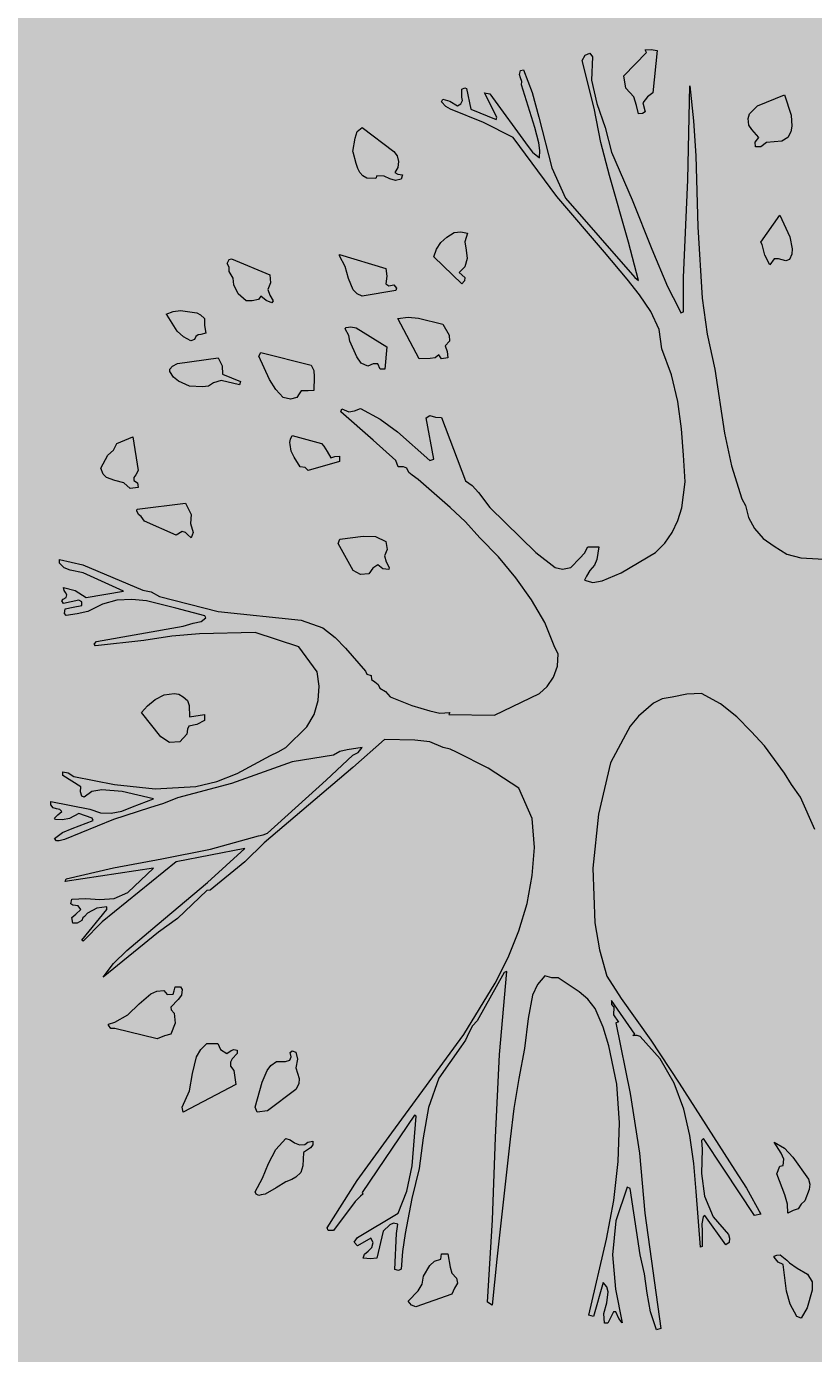
# Model space of a CAD drawing. Units: inches. Extents: x 84 to 1044, y -280 to 906.
# Tile 70 of 105: x 705 to 719, y 408 to 432. Entities that reach past the tile are written whole.
import ezdxf

# ---------------------------------------------------------------- set-up
doc = ezdxf.new("R2010")
doc.units = ezdxf.units.IN
doc.layers.add('A-ANNO-DIMS', color=2, linetype='Continuous', lineweight=18)
doc.layers.add('L-PLNT', color=114, linetype='Continuous', lineweight=15)
doc.layers.add('L-PLNT-PATT', color=9, linetype='Continuous', lineweight=9, true_color=0xafd9aa)
doc.styles.get("Standard").update_dxf_attribs({"font": 'arial.ttf'})
doc.dimstyles.get("Standard").update_dxf_attribs({"dimtxt": 0.18, "dimasz": 0.18, "dimexe": 0.18, "dimexo": 0.0625, "dimgap": 0.09, "dimtad": 0, "dimtih": 1, "dimtoh": 1, "dimdec": 4, "dimzin": 0, "dimdsep": 46, "dimtxsty": 'Standard', "dimcen": 0.09, "dimadec": 0, "dimazin": 0, "dimtfac": 1, "dimtdec": 4, "dimtofl": 0, "dimtmove": 0, "dimatfit": 3, "dimfxl": 1, "dimtolj": 1, "dimtzin": 0, "dimarcsym": 0})

# ---------------------------------------------------------------- blocks, each defined once
blk = doc.blocks.new('A$C37E508DF')
for p, q in [((0.6329, 1.5111), (0.6367, 1.5175)), ((0.6367, 1.5175), (0.6423, 1.5201)), ((0.6423, 1.5201), (0.6453, 1.5158)), ((0.6826, 1.493), (0.7096, 1.5209)), ((0.7083, 1.5239), (0.7152, 1.5244)), ((0.7096, 1.5209), (0.7083, 1.5239)), ((0.7152, 1.5244), (0.7225, 1.5231)), ((0.7225, 1.5231), (0.7174, 1.4729)), ((0.6475, 1.4545), (0.6329, 1.5111)), ((0.6453, 1.5158), (0.644, 1.4879)), ((0.5583, 1.4948), (0.5596, 1.4995)), ((0.5596, 1.4905), (0.5583, 1.4948)), ((0.5596, 1.4995), (0.563, 1.5003)), ((0.5613, 1.4862), (0.5596, 1.4905)), ((0.5608, 1.4823), (0.5613, 1.4862)), ((0.563, 1.5003), (0.5737, 1.4733)), ((0.644, 1.4879), (0.6505, 1.46)), ((0.6852, 1.4785), (0.6826, 1.493)), ((0.4897, 1.4772), (0.4935, 1.4789)), ((0.4897, 1.4678), (0.4897, 1.4772)), ((0.4935, 1.4789), (0.4952, 1.478)), ((0.4952, 1.478), (0.5004, 1.4532)), ((0.5313, 1.4437), (0.5167, 1.4729)), ((0.5167, 1.4729), (0.5231, 1.4716)), ((0.5231, 1.4716), (0.5686, 1.409)), ((0.5767, 1.4317), (0.5608, 1.4823)), ((0.5737, 1.4733), (0.5814, 1.4437)), ((0.6946, 1.4682), (0.6852, 1.4785)), ((0.7174, 1.4729), (0.7109, 1.4682)), ((0.7589, 1.3691), (0.7615, 1.481)), ((0.7615, 1.481), (0.7658, 1.4395)), ((0.8421, 1.4575), (0.8739, 1.4703)), ((0.8739, 1.4703), (0.882, 1.4463)), ((0.4657, 1.4622), (0.4669, 1.4652)), ((0.4708, 1.4566), (0.4657, 1.4622)), ((0.4669, 1.4652), (0.4755, 1.463)), ((0.4764, 1.4532), (0.4708, 1.4566)), ((0.4755, 1.463), (0.4845, 1.4575)), ((0.4845, 1.4575), (0.4884, 1.4596)), ((0.4884, 1.4596), (0.4905, 1.4635)), ((0.4905, 1.4635), (0.4897, 1.4678)), ((0.6552, 1.4137), (0.6475, 1.4545)), ((0.6505, 1.46), (0.6603, 1.4317)), ((0.6976, 1.4579), (0.6946, 1.4682)), ((0.7002, 1.4476), (0.6976, 1.4579)), ((0.7109, 1.4682), (0.7053, 1.4609)), ((0.7053, 1.4609), (0.7083, 1.4502)), ((0.8357, 1.451), (0.8421, 1.4575)), ((0.5154, 1.4373), (0.4764, 1.4532)), ((0.5004, 1.4532), (0.5308, 1.4412)), ((0.5308, 1.4412), (0.5313, 1.4437)), ((0.5814, 1.4437), (0.5969, 1.3833)), ((0.7049, 1.448), (0.7002, 1.4476)), ((0.7083, 1.4502), (0.7049, 1.448)), ((0.7658, 1.4395), (0.7684, 1.3979)), ((0.831, 1.4424), (0.8323, 1.4476)), ((0.8318, 1.4343), (0.831, 1.4424)), ((0.8323, 1.4476), (0.8357, 1.451)), ((0.882, 1.4463), (0.8829, 1.433)), ((0.3628, 1.4189), (0.3649, 1.4266)), ((0.3649, 1.4266), (0.3709, 1.4317)), ((0.3709, 1.4317), (0.4086, 1.403)), ((0.551, 1.4197), (0.5154, 1.4373)), ((0.5814, 1.4133), (0.5767, 1.4317)), ((0.6603, 1.4317), (0.668, 1.4021)), ((0.8353, 1.4292), (0.8318, 1.4343)), ((0.8434, 1.4197), (0.8353, 1.4292)), ((0.8816, 1.4262), (0.8781, 1.4197)), ((0.8829, 1.433), (0.8816, 1.4262)), ((0.3598, 1.403), (0.3628, 1.4189)), ((0.6029, 1.3494), (0.551, 1.4197)), ((0.5686, 1.409), (0.5741, 1.4021)), ((0.5827, 1.4043), (0.5814, 1.4133)), ((0.6655, 1.3743), (0.6552, 1.4137)), ((0.8391, 1.4141), (0.8434, 1.4197)), ((0.8395, 1.4086), (0.8391, 1.4141)), ((0.846, 1.4086), (0.8395, 1.4086)), ((0.8528, 1.4137), (0.846, 1.4086)), ((0.8619, 1.4146), (0.8528, 1.4137)), ((0.8709, 1.4154), (0.8619, 1.4146)), ((0.8781, 1.4197), (0.8709, 1.4154)), ((0.3602, 1.4021), (0.3598, 1.403)), ((0.364, 1.3888), (0.3602, 1.4021)), ((0.4086, 1.403), (0.4125, 1.3979)), ((0.4125, 1.3979), (0.4142, 1.391)), ((0.4142, 1.391), (0.4134, 1.3837)), ((0.5741, 1.4021), (0.5823, 1.3953)), ((0.5823, 1.3953), (0.5827, 1.4043)), ((0.668, 1.4021), (0.6925, 1.3455)), ((0.7684, 1.3979), (0.771, 1.3134)), ((0.3657, 1.3828), (0.364, 1.3888)), ((0.3683, 1.3781), (0.3657, 1.3828)), ((0.3718, 1.3738), (0.3683, 1.3781)), ((0.4134, 1.3837), (0.4099, 1.3781)), ((0.4099, 1.3781), (0.4134, 1.376)), ((0.4134, 1.376), (0.4189, 1.3751)), ((0.4189, 1.3751), (0.4176, 1.37)), ((0.5969, 1.3833), (0.6132, 1.3472)), ((0.3765, 1.3713), (0.3718, 1.3738)), ((0.3872, 1.3708), (0.3765, 1.3713)), ((0.3885, 1.3738), (0.3872, 1.3708)), ((0.3971, 1.3734), (0.3885, 1.3738)), ((0.4039, 1.3704), (0.3971, 1.3734)), ((0.4108, 1.3683), (0.4039, 1.3704)), ((0.4176, 1.37), (0.4108, 1.3683)), ((0.6882, 1.2949), (0.6655, 1.3743)), ((0.7538, 1.2529), (0.7589, 1.3691)), ((0.6595, 1.2829), (0.6029, 1.3494)), ((0.6132, 1.3472), (0.6959, 1.2529)), ((0.6925, 1.3455), (0.7161, 1.2868)), ((0.771, 1.3134), (0.7761, 1.2285)), ((0.846, 1.2949), (0.8687, 1.3271)), ((0.8687, 1.3271), (0.8803, 1.3014)), ((0.4648, 1.2945), (0.4717, 1.3009)), ((0.4717, 1.3009), (0.4807, 1.3065)), ((0.4807, 1.3065), (0.4884, 1.3074)), ((0.4884, 1.3074), (0.4965, 1.3057)), ((0.4965, 1.3057), (0.4935, 1.2954)), ((0.8803, 1.3014), (0.8833, 1.2872)), ((0.3439, 1.2804), (0.3992, 1.2636)), ((0.3439, 1.2787), (0.3439, 1.2804)), ((0.4562, 1.2774), (0.4597, 1.2868)), ((0.4597, 1.2868), (0.4648, 1.2945)), ((0.4935, 1.2954), (0.4948, 1.2855)), ((0.4948, 1.2855), (0.4961, 1.2756)), ((0.6865, 1.2508), (0.6595, 1.2829)), ((0.7002, 1.2495), (0.6882, 1.2949)), ((0.7161, 1.2868), (0.7349, 1.2422)), ((0.8473, 1.2924), (0.846, 1.2949)), ((0.8507, 1.2795), (0.8473, 1.2924)), ((0.8829, 1.2808), (0.8799, 1.2744)), ((0.8833, 1.2872), (0.8829, 1.2808)), ((0.2101, 1.2696), (0.2127, 1.2744)), ((0.2127, 1.2654), (0.2101, 1.2696)), ((0.2127, 1.2744), (0.2152, 1.2752)), ((0.2127, 1.2602), (0.2127, 1.2654)), ((0.2152, 1.2752), (0.2611, 1.2559)), ((0.3507, 1.2662), (0.3439, 1.2787)), ((0.3546, 1.2516), (0.3507, 1.2662)), ((0.4897, 1.2452), (0.4562, 1.2774)), ((0.4935, 1.2658), (0.4867, 1.2589)), ((0.4961, 1.2756), (0.4935, 1.2658)), ((0.8567, 1.2679), (0.8507, 1.2795)), ((0.8619, 1.2752), (0.8567, 1.2679)), ((0.867, 1.2752), (0.8619, 1.2752)), ((0.8713, 1.2739), (0.867, 1.2752)), ((0.8756, 1.2726), (0.8713, 1.2739)), ((0.8799, 1.2744), (0.8756, 1.2726)), ((0.2174, 1.2521), (0.2127, 1.2602)), ((0.2182, 1.2443), (0.2174, 1.2521)), ((0.2611, 1.2559), (0.262, 1.2465)), ((0.3602, 1.2383), (0.3546, 1.2516)), ((0.3992, 1.2636), (0.4005, 1.2546)), ((0.4005, 1.2546), (0.3992, 1.2452)), ((0.4867, 1.2589), (0.4935, 1.2529)), ((0.4931, 1.2491), (0.4897, 1.2452)), ((0.4935, 1.2529), (0.4931, 1.2491)), ((0.7015, 1.2323), (0.6865, 1.2508)), ((0.6959, 1.2529), (0.7002, 1.2495)), ((0.7538, 1.2122), (0.7538, 1.2529)), ((0.2234, 1.2336), (0.2182, 1.2443)), ((0.2328, 1.2251), (0.2234, 1.2336)), ((0.262, 1.2465), (0.2586, 1.2388)), ((0.2586, 1.2388), (0.2611, 1.2319)), ((0.3649, 1.2336), (0.3602, 1.2383)), ((0.3709, 1.2306), (0.3649, 1.2336)), ((0.4112, 1.2375), (0.3709, 1.2306)), ((0.3992, 1.2452), (0.4026, 1.2431)), ((0.4026, 1.2431), (0.4086, 1.2443)), ((0.4086, 1.2443), (0.4121, 1.2401)), ((0.4121, 1.2401), (0.4112, 1.2375)), ((0.7349, 1.2422), (0.7482, 1.216)), ((0.2401, 1.2251), (0.2328, 1.2251)), ((0.2474, 1.2268), (0.2401, 1.2251)), ((0.2504, 1.2306), (0.2474, 1.2268)), ((0.2568, 1.2255), (0.2504, 1.2306)), ((0.2633, 1.2229), (0.2568, 1.2255)), ((0.2611, 1.2319), (0.265, 1.2251)), ((0.265, 1.2251), (0.2633, 1.2229)), ((0.7148, 1.2126), (0.7015, 1.2323)), ((0.7761, 1.2285), (0.7821, 1.1856)), ((0.1376, 1.2092), (0.1458, 1.2126)), ((0.1389, 1.2079), (0.1376, 1.2092)), ((0.1505, 1.189), (0.1389, 1.2079)), ((0.1458, 1.2126), (0.1548, 1.2135)), ((0.1548, 1.2135), (0.1741, 1.2109)), ((0.1741, 1.2109), (0.1784, 1.2083)), ((0.1784, 1.2083), (0.1831, 1.204)), ((0.1831, 1.204), (0.1831, 1.1959)), ((0.4134, 1.204), (0.4258, 1.2058)), ((0.4391, 1.156), (0.4134, 1.204)), ((0.4258, 1.2058), (0.4382, 1.2045)), ((0.4382, 1.2045), (0.4669, 1.1972)), ((0.7246, 1.1908), (0.7148, 1.2126)), ((0.7482, 1.216), (0.7508, 1.2109)), ((0.7508, 1.2109), (0.7538, 1.2122)), ((0.1582, 1.1822), (0.1505, 1.189)), ((0.1788, 1.1852), (0.1758, 1.1847)), ((0.1848, 1.1865), (0.1788, 1.1852)), ((0.1831, 1.1959), (0.1848, 1.1865)), ((0.3507, 1.1916), (0.352, 1.1933)), ((0.355, 1.1839), (0.3507, 1.1916)), ((0.352, 1.1933), (0.3576, 1.1942)), ((0.3576, 1.1942), (0.364, 1.1929)), ((0.364, 1.1929), (0.4005, 1.1702)), ((0.4669, 1.1972), (0.4747, 1.1843)), ((0.7281, 1.168), (0.7246, 1.1908)), ((0.7821, 1.1856), (0.7911, 1.1436)), ((0.1668, 1.1775), (0.1582, 1.1822)), ((0.1711, 1.1792), (0.1668, 1.1775)), ((0.1728, 1.1826), (0.1711, 1.1792)), ((0.1758, 1.1847), (0.1728, 1.1826)), ((0.3563, 1.177), (0.355, 1.1839)), ((0.3645, 1.1586), (0.3563, 1.177)), ((0.4005, 1.1702), (0.3979, 1.1436)), ((0.4751, 1.177), (0.47, 1.1714)), ((0.47, 1.1714), (0.4721, 1.1646)), ((0.4747, 1.1843), (0.4751, 1.177)), ((0.1509, 1.1504), (0.1994, 1.1573)), ((0.1994, 1.1573), (0.2041, 1.1479)), ((0.2478, 1.1594), (0.2504, 1.1637)), ((0.2607, 1.1316), (0.2478, 1.1594)), ((0.2504, 1.1637), (0.3104, 1.1487)), ((0.37, 1.1509), (0.3645, 1.1586)), ((0.4519, 1.1564), (0.4391, 1.156)), ((0.458, 1.1573), (0.4519, 1.1564)), ((0.4622, 1.1607), (0.458, 1.1573)), ((0.4657, 1.156), (0.4622, 1.1607)), ((0.473, 1.1573), (0.4657, 1.156)), ((0.4721, 1.1646), (0.473, 1.1573)), ((0.7396, 1.1371), (0.7281, 1.168)), ((0.1419, 1.1436), (0.1449, 1.1474)), ((0.1419, 1.141), (0.1419, 1.1436)), ((0.1462, 1.1342), (0.1419, 1.141)), ((0.1449, 1.1474), (0.1509, 1.1504)), ((0.2041, 1.1479), (0.2045, 1.138)), ((0.2045, 1.138), (0.226, 1.129)), ((0.3104, 1.1487), (0.3134, 1.1423)), ((0.3134, 1.1423), (0.3139, 1.1346)), ((0.3778, 1.1474), (0.37, 1.1509)), ((0.3842, 1.15), (0.3778, 1.1474)), ((0.3898, 1.15), (0.3842, 1.15)), ((0.3923, 1.1436), (0.3898, 1.15)), ((0.3979, 1.1436), (0.3923, 1.1436)), ((0.7911, 1.1436), (0.8027, 1.0677)), ((0.1522, 1.1294), (0.1462, 1.1342)), ((0.1655, 1.1234), (0.1522, 1.1294)), ((0.181, 1.1226), (0.1655, 1.1234)), ((0.1878, 1.1234), (0.181, 1.1226)), ((0.1938, 1.1273), (0.1878, 1.1234)), ((0.2032, 1.1303), (0.1938, 1.1273)), ((0.2247, 1.1251), (0.2032, 1.1303)), ((0.226, 1.129), (0.2247, 1.1251)), ((0.268, 1.1196), (0.2607, 1.1316)), ((0.3139, 1.1346), (0.3134, 1.1183)), ((0.7469, 1.1054), (0.7396, 1.1371)), ((0.277, 1.1101), (0.268, 1.1196)), ((0.2856, 1.108), (0.277, 1.1101)), ((0.2933, 1.1101), (0.2856, 1.108)), ((0.2959, 1.1144), (0.2933, 1.1101)), ((0.2984, 1.1179), (0.2959, 1.1144)), ((0.3066, 1.1179), (0.2984, 1.1179)), ((0.3134, 1.1183), (0.3066, 1.1179)), ((0.3456, 1.093), (0.3469, 1.0964)), ((0.3842, 1.0591), (0.3456, 1.093)), ((0.3469, 1.0964), (0.355, 1.093)), ((0.355, 1.093), (0.3619, 1.0943)), ((0.3619, 1.0943), (0.3692, 1.0968)), ((0.3692, 1.0968), (0.3923, 1.0844)), ((0.7512, 1.0728), (0.7469, 1.1054)), ((0.3923, 1.0844), (0.4129, 1.069)), ((0.4472, 1.0857), (0.4515, 1.0887)), ((0.4562, 1.0364), (0.4472, 1.0857)), ((0.4515, 1.0887), (0.4584, 1.0865)), ((0.4584, 1.0865), (0.4657, 1.0861)), ((0.4657, 1.0861), (0.4939, 1.0107)), ((0.0789, 1.0552), (0.0978, 1.063)), ((0.0978, 1.063), (0.1042, 1.0231)), ((0.2847, 1.0565), (0.2856, 1.0604)), ((0.2856, 1.0604), (0.2877, 1.0647)), ((0.2877, 1.0647), (0.3224, 1.0552)), ((0.4112, 1.0351), (0.3842, 1.0591)), ((0.4129, 1.069), (0.4515, 1.0351)), ((0.7538, 1.0415), (0.7512, 1.0728)), ((0.8027, 1.0677), (0.8108, 1.0287)), ((0.0682, 1.0415), (0.0746, 1.0475)), ((0.0746, 1.0475), (0.0789, 1.0552)), ((0.2851, 1.054), (0.2847, 1.0565)), ((0.2864, 1.0463), (0.2851, 1.054)), ((0.2899, 1.039), (0.2864, 1.0463)), ((0.3224, 1.0552), (0.3255, 1.0522)), ((0.3255, 1.0522), (0.3293, 1.0458)), ((0.3293, 1.0458), (0.3336, 1.0381)), ((0.0596, 1.0257), (0.0682, 1.0415)), ((0.2972, 1.0274), (0.2899, 1.039)), ((0.3032, 1.0265), (0.2972, 1.0274)), ((0.3439, 1.0338), (0.3066, 1.0231)), ((0.3336, 1.0381), (0.3383, 1.0398)), ((0.3383, 1.0398), (0.3439, 1.0402)), ((0.3439, 1.0402), (0.3439, 1.0338)), ((0.4138, 1.0274), (0.4112, 1.0351)), ((0.4202, 1.0274), (0.4138, 1.0274)), ((0.4241, 1.0257), (0.4202, 1.0274)), ((0.4515, 1.0351), (0.4562, 1.0364)), ((0.7559, 1.0098), (0.7538, 1.0415)), ((0.8108, 1.0287), (0.8233, 0.9892)), ((0.0626, 1.0188), (0.0596, 1.0257)), ((0.0665, 1.0149), (0.0626, 1.0188)), ((0.0763, 1.0111), (0.0665, 1.0149)), ((0.1012, 1.018), (0.099, 1.0149)), ((0.099, 1.0149), (0.099, 1.0111)), ((0.1042, 1.0231), (0.1012, 1.018)), ((0.3066, 1.0231), (0.3032, 1.0265)), ((0.4267, 1.0209), (0.4241, 1.0257)), ((0.4305, 1.0175), (0.4267, 1.0209)), ((0.4378, 1.0124), (0.4305, 1.0175)), ((0.476, 0.9789), (0.4378, 1.0124)), ((0.087, 1.0085), (0.0763, 1.0111)), ((0.0948, 1.0016), (0.087, 1.0085)), ((0.1042, 1.0029), (0.0948, 1.0016)), ((0.099, 1.0111), (0.1033, 1.0085)), ((0.1033, 1.0085), (0.1042, 1.0029)), ((0.4939, 1.0107), (0.5021, 1.0051)), ((0.5021, 1.0051), (0.5094, 0.9969)), ((0.5094, 0.9969), (0.5231, 0.9789)), ((0.7516, 0.9785), (0.7559, 1.0098)), ((0.1029, 0.9772), (0.1604, 0.9841)), ((0.1604, 0.9841), (0.1672, 0.9708)), ((0.8233, 0.9892), (0.8275, 0.9815)), ((0.8275, 0.9815), (0.8314, 0.9673)), ((0.1025, 0.9751), (0.1029, 0.9772)), ((0.1046, 0.9708), (0.1025, 0.9751)), ((0.1076, 0.9682), (0.1046, 0.9708)), ((0.1119, 0.9626), (0.1076, 0.9682)), ((0.1672, 0.9708), (0.1664, 0.9601)), ((0.4939, 0.9618), (0.476, 0.9789)), ((0.5231, 0.9789), (0.578, 0.9253)), ((0.7469, 0.9635), (0.7516, 0.9785)), ((0.8314, 0.9673), (0.8383, 0.954)), ((0.1496, 0.9463), (0.1119, 0.9626)), ((0.1565, 0.9506), (0.1496, 0.9463)), ((0.1604, 0.9493), (0.1565, 0.9506)), ((0.1629, 0.9468), (0.1604, 0.9493)), ((0.1664, 0.9601), (0.1698, 0.9493)), ((0.1698, 0.9493), (0.1672, 0.9429)), ((0.5111, 0.9429), (0.4939, 0.9618)), ((0.7315, 0.9365), (0.7401, 0.9493)), ((0.7401, 0.9493), (0.7469, 0.9635)), ((0.8383, 0.954), (0.8486, 0.942)), ((0.1672, 0.9429), (0.1629, 0.9468)), ((0.3426, 0.936), (0.3443, 0.9412)), ((0.3602, 0.9039), (0.3426, 0.936)), ((0.3443, 0.9412), (0.3722, 0.9451)), ((0.3722, 0.9451), (0.3868, 0.9446)), ((0.3868, 0.9446), (0.3992, 0.9386)), ((0.3992, 0.9386), (0.4009, 0.9292)), ((0.5334, 0.9202), (0.5111, 0.9429)), ((0.6359, 0.9245), (0.6397, 0.9322)), ((0.6397, 0.9322), (0.653, 0.9322)), ((0.653, 0.9322), (0.6505, 0.9172)), ((0.7203, 0.9253), (0.7315, 0.9365)), ((0.8486, 0.942), (0.8619, 0.933)), ((0.8619, 0.933), (0.8769, 0.9236)), ((0.0103, 0.9129), (0.0103, 0.9172)), ((0.0103, 0.9172), (0.0382, 0.9107)), ((0.4009, 0.9292), (0.3975, 0.9215)), ((0.3975, 0.9215), (0.3996, 0.9142)), ((0.554, 0.8953), (0.5334, 0.9202)), ((0.578, 0.9253), (0.6011, 0.9077)), ((0.6196, 0.9077), (0.6303, 0.9189)), ((0.6303, 0.9189), (0.6359, 0.9245)), ((0.6505, 0.9172), (0.6479, 0.9103)), ((0.6796, 0.9013), (0.7203, 0.9253)), ((0.8769, 0.9236), (0.8936, 0.9193)), ((0.8936, 0.9193), (0.9279, 0.9172)), ((0.0159, 0.9073), (0.0103, 0.9129)), ((0.0232, 0.9043), (0.0159, 0.9073)), ((0.0386, 0.9013), (0.0232, 0.9043)), ((0.0382, 0.9107), (0.1098, 0.8807)), ((0.0866, 0.8794), (0.0386, 0.9013)), ((0.3692, 0.8992), (0.3602, 0.9039)), ((0.3838, 0.9069), (0.379, 0.9)), ((0.3898, 0.9107), (0.3838, 0.9069)), ((0.3958, 0.906), (0.3898, 0.9107)), ((0.4026, 0.9052), (0.3958, 0.906)), ((0.3996, 0.9142), (0.4031, 0.9077)), ((0.4031, 0.9077), (0.4026, 0.9052)), ((0.6011, 0.9077), (0.6097, 0.9056)), ((0.6097, 0.9056), (0.6196, 0.9077)), ((0.6423, 0.9039), (0.6384, 0.8974)), ((0.6479, 0.9103), (0.6423, 0.9039)), ((0.6569, 0.8919), (0.6796, 0.9013)), ((0.379, 0.9), (0.3692, 0.8992)), ((0.5728, 0.8691), (0.554, 0.8953)), ((0.6384, 0.8974), (0.6359, 0.8927)), ((0.6359, 0.8927), (0.6457, 0.8897)), ((0.6457, 0.8897), (0.6569, 0.8919)), ((0.0133, 0.8679), (0.015, 0.87)), ((0.015, 0.87), (0.0184, 0.8717)), ((0.0159, 0.8803), (0.0154, 0.8837)), ((0.0154, 0.8837), (0.0292, 0.8803)), ((0.0176, 0.8777), (0.0159, 0.8803)), ((0.0193, 0.8752), (0.0176, 0.8777)), ((0.0184, 0.8717), (0.0193, 0.8752)), ((0.0292, 0.8803), (0.0424, 0.8717)), ((0.0424, 0.8717), (0.0866, 0.8794)), ((0.0965, 0.8696), (0.0789, 0.8687)), ((0.1141, 0.8679), (0.0965, 0.8696)), ((0.1098, 0.8807), (0.1196, 0.8786)), ((0.1196, 0.8786), (0.1295, 0.873)), ((0.1295, 0.873), (0.1994, 0.8554)), ((0.5887, 0.8421), (0.5728, 0.8691)), ((0.0154, 0.8649), (0.0133, 0.8679)), ((0.0334, 0.8687), (0.0154, 0.8649)), ((0.0163, 0.8529), (0.0171, 0.8584)), ((0.0171, 0.8584), (0.0266, 0.8602)), ((0.0266, 0.8602), (0.0369, 0.8623)), ((0.0442, 0.8554), (0.0317, 0.8524)), ((0.0369, 0.8666), (0.0334, 0.8687)), ((0.0369, 0.8623), (0.0369, 0.8666)), ((0.0617, 0.864), (0.0442, 0.8554)), ((0.0789, 0.8687), (0.0617, 0.864)), ((0.1492, 0.8593), (0.1141, 0.8679)), ((0.1835, 0.8499), (0.1492, 0.8593)), ((0.1994, 0.8554), (0.2984, 0.8447)), ((0.0184, 0.8503), (0.0163, 0.8529)), ((0.0317, 0.8524), (0.0184, 0.8503)), ((0.0545, 0.8194), (0.1578, 0.8378)), ((0.1578, 0.8378), (0.1698, 0.8413)), ((0.1698, 0.8413), (0.1792, 0.8434)), ((0.1792, 0.8434), (0.1848, 0.8477)), ((0.1848, 0.8477), (0.1835, 0.8499)), ((0.2984, 0.8447), (0.3242, 0.8357)), ((0.6007, 0.8125), (0.5887, 0.8421)), ((0.1441, 0.8258), (0.1111, 0.8207)), ((0.1771, 0.8288), (0.1441, 0.8258)), ((0.2436, 0.8301), (0.1771, 0.8288)), ((0.2954, 0.813), (0.2436, 0.8301)), ((0.3242, 0.8357), (0.3387, 0.8241)), ((0.3387, 0.8241), (0.3512, 0.8117)), ((0.0519, 0.8164), (0.0545, 0.8194)), ((0.0532, 0.8143), (0.0519, 0.8164)), ((0.1111, 0.8207), (0.0532, 0.8143)), ((0.3173, 0.7834), (0.2954, 0.813)), ((0.3512, 0.8117), (0.3748, 0.7842)), ((0.6046, 0.8048), (0.6007, 0.8125)), ((0.599, 0.777), (0.6037, 0.7903)), ((0.6037, 0.7903), (0.6046, 0.8048)), ((0.3199, 0.7662), (0.3173, 0.7834)), ((0.3748, 0.7842), (0.3765, 0.7804)), ((0.3765, 0.7804), (0.3816, 0.7791)), ((0.3816, 0.7791), (0.382, 0.7744)), ((0.382, 0.7744), (0.3859, 0.7714)), ((0.5913, 0.7658), (0.599, 0.777)), ((0.3186, 0.7491), (0.3199, 0.7662)), ((0.3859, 0.7714), (0.3902, 0.7684)), ((0.3902, 0.7684), (0.3919, 0.7641)), ((0.3919, 0.7641), (0.3988, 0.7598)), ((0.3988, 0.7598), (0.4043, 0.7538)), ((0.5823, 0.7577), (0.5913, 0.7658)), ((0.1081, 0.7349), (0.1153, 0.7427)), ((0.1153, 0.7427), (0.1244, 0.7504)), ((0.1244, 0.7504), (0.1351, 0.7559)), ((0.1351, 0.7559), (0.1471, 0.7577)), ((0.1471, 0.7577), (0.1527, 0.7568)), ((0.1527, 0.7568), (0.1578, 0.7538)), ((0.1578, 0.7538), (0.1629, 0.7491)), ((0.1629, 0.7491), (0.1651, 0.7431)), ((0.1651, 0.7431), (0.1655, 0.7298)), ((0.3139, 0.7324), (0.3186, 0.7491)), ((0.4043, 0.7538), (0.4301, 0.7431)), ((0.4301, 0.7431), (0.4515, 0.7371)), ((0.5287, 0.7319), (0.5823, 0.7577)), ((0.7182, 0.7461), (0.7002, 0.7307)), ((0.7285, 0.7512), (0.7182, 0.7461)), ((0.7401, 0.7534), (0.7285, 0.7512)), ((0.7577, 0.7568), (0.7401, 0.7534)), ((0.7752, 0.7577), (0.7577, 0.7568)), ((0.798, 0.7452), (0.7752, 0.7577)), ((0.8173, 0.7298), (0.798, 0.7452)), ((0.1312, 0.7058), (0.1081, 0.7349)), ((0.1655, 0.7298), (0.1831, 0.7324)), ((0.1831, 0.7324), (0.1831, 0.7255)), ((0.3049, 0.7178), (0.3139, 0.7324)), ((0.4515, 0.7371), (0.4635, 0.7341)), ((0.4635, 0.7341), (0.4755, 0.7349)), ((0.4755, 0.7349), (0.4742, 0.7324)), ((0.4742, 0.7324), (0.5287, 0.7319)), ((0.7002, 0.7307), (0.6903, 0.7186)), ((0.8344, 0.7122), (0.8173, 0.7298)), ((0.1629, 0.7152), (0.1621, 0.7092)), ((0.1646, 0.7186), (0.1629, 0.7152)), ((0.1741, 0.7208), (0.1646, 0.7186)), ((0.1831, 0.7255), (0.1741, 0.7208)), ((0.28, 0.6933), (0.3049, 0.7178)), ((0.6903, 0.7186), (0.6818, 0.7032)), ((0.8503, 0.6951), (0.8344, 0.7122)), ((0.1415, 0.6994), (0.1312, 0.7058)), ((0.1539, 0.7002), (0.1415, 0.6994)), ((0.1621, 0.7092), (0.1539, 0.7002)), ((0.3975, 0.7028), (0.3598, 0.6693)), ((0.4339, 0.7019), (0.3975, 0.7028)), ((0.4515, 0.7002), (0.4339, 0.7019)), ((0.4674, 0.6933), (0.4515, 0.7002)), ((0.6818, 0.7032), (0.6667, 0.6749)), ((0.2221, 0.6625), (0.262, 0.6839)), ((0.262, 0.6839), (0.271, 0.6882)), ((0.271, 0.6882), (0.28, 0.6933)), ((0.337, 0.6843), (0.2877, 0.6762)), ((0.328, 0.6543), (0.3598, 0.6843)), ((0.3443, 0.6886), (0.337, 0.6843)), ((0.3533, 0.6903), (0.3443, 0.6886)), ((0.3709, 0.6933), (0.3533, 0.6903)), ((0.3598, 0.6843), (0.3662, 0.6873)), ((0.3662, 0.6873), (0.3709, 0.6933)), ((0.476, 0.6912), (0.4674, 0.6933)), ((0.4832, 0.6878), (0.476, 0.6912)), ((0.521, 0.6685), (0.4832, 0.6878)), ((0.8739, 0.6629), (0.8503, 0.6951)), ((0.0146, 0.6599), (0.0146, 0.6642)), ((0.0146, 0.6642), (0.0206, 0.6633)), ((0.2877, 0.6762), (0.2152, 0.6505)), ((0.3598, 0.6693), (0.2543, 0.5797)), ((0.5578, 0.6449), (0.521, 0.6685)), ((0.6667, 0.6749), (0.6526, 0.614)), ((0.036, 0.6466), (0.0146, 0.6599)), ((0.0206, 0.6633), (0.0274, 0.6586)), ((0.0274, 0.6586), (0.0759, 0.6492)), ((0.0759, 0.6492), (0.1244, 0.644)), ((0.2152, 0.6505), (0.1509, 0.6333)), ((0.1728, 0.647), (0.1977, 0.6526)), ((0.1977, 0.6526), (0.2221, 0.6625)), ((0.2581, 0.5913), (0.328, 0.6543)), ((0.8824, 0.6492), (0.8739, 0.6629)), ((0.8932, 0.6342), (0.8824, 0.6492)), ((0.0356, 0.6406), (0.036, 0.6466)), ((0.0369, 0.6355), (0.0356, 0.6406)), ((0.0399, 0.6342), (0.0369, 0.6355)), ((0.0489, 0.641), (0.0399, 0.6342)), ((0.0609, 0.6428), (0.0489, 0.641)), ((0.0853, 0.641), (0.0609, 0.6428)), ((0.1226, 0.632), (0.0853, 0.641)), ((0.0973, 0.6226), (0.1226, 0.632)), ((0.1244, 0.644), (0.1728, 0.647)), ((0.1509, 0.6333), (0.1342, 0.6265)), ((0.5737, 0.6089), (0.5578, 0.6449)), ((0.9103, 0.5956), (0.8932, 0.6342)), ((0, 0.629), (0.0467, 0.62)), ((0, 0.6252), (0, 0.629)), ((0.003, 0.6213), (0, 0.6252)), ((0.0069, 0.6204), (0.003, 0.6213)), ((0.0107, 0.6196), (0.0069, 0.6204)), ((0.0086, 0.6132), (0.0133, 0.617)), ((0.0133, 0.617), (0.0107, 0.6196)), ((0.0467, 0.62), (0.0592, 0.6153)), ((0.072, 0.6149), (0.0849, 0.6175)), ((0.1175, 0.6213), (0.0746, 0.6076)), ((0.0849, 0.6175), (0.0973, 0.6226)), ((0.1342, 0.6265), (0.1175, 0.6213)), ((0.0047, 0.6093), (0.0086, 0.6132)), ((0.0056, 0.6076), (0.0047, 0.6093)), ((0.0141, 0.6072), (0.0056, 0.6076)), ((0.0223, 0.6089), (0.0141, 0.6072)), ((0.0746, 0.6076), (0.0163, 0.5836)), ((0.0334, 0.6145), (0.0223, 0.6089)), ((0.0257, 0.5969), (0.0506, 0.6063)), ((0.0416, 0.6119), (0.0334, 0.6145)), ((0.0493, 0.6093), (0.0416, 0.6119)), ((0.0506, 0.6063), (0.0493, 0.6093)), ((0.0592, 0.6153), (0.072, 0.6149)), ((0.5763, 0.5741), (0.5737, 0.6089)), ((0.6526, 0.614), (0.6457, 0.5497)), ((0.0047, 0.5849), (0.0141, 0.5921)), ((0.0069, 0.5823), (0.0047, 0.5849)), ((0.0141, 0.5921), (0.0257, 0.5969)), ((0.1904, 0.5724), (0.2474, 0.5879)), ((0.2474, 0.5879), (0.253, 0.5892)), ((0.253, 0.5892), (0.2581, 0.5913)), ((0.0099, 0.5823), (0.0069, 0.5823)), ((0.0163, 0.5836), (0.0099, 0.5823)), ((0.1325, 0.5608), (0.1904, 0.5724)), ((0.2311, 0.5729), (0.1496, 0.557)), ((0.1869, 0.5325), (0.2311, 0.5729)), ((0.2543, 0.5797), (0.2311, 0.557)), ((0.5737, 0.5407), (0.5763, 0.5741)), ((0.1496, 0.557), (0.0613, 0.4858)), ((0.0746, 0.5501), (0.1325, 0.5608)), ((0.2311, 0.557), (0.1899, 0.5235)), ((0.1226, 0.5497), (0.0171, 0.5338)), ((0.0184, 0.5368), (0.0746, 0.5501)), ((0.0917, 0.5205), (0.1226, 0.5497)), ((0.5677, 0.5077), (0.5737, 0.5407)), ((0.6457, 0.5497), (0.6483, 0.4845)), ((0.0171, 0.5338), (0.0184, 0.5368)), ((0.1269, 0.482), (0.1869, 0.5325)), ((0.1861, 0.5231), (0.1509, 0.4897)), ((0.1899, 0.5235), (0.1861, 0.5231)), ((0.024, 0.5072), (0.0253, 0.5128)), ((0.0262, 0.5055), (0.024, 0.5072)), ((0.0253, 0.5128), (0.042, 0.5133)), ((0.042, 0.5133), (0.0587, 0.5124)), ((0.0587, 0.5124), (0.0755, 0.5133)), ((0.0755, 0.5133), (0.0917, 0.5205)), ((0.5578, 0.4751), (0.5677, 0.5077)), ((0.0253, 0.491), (0.03, 0.4948)), ((0.0262, 0.4841), (0.0253, 0.491)), ((0.0326, 0.5047), (0.0262, 0.5055)), ((0.03, 0.4948), (0.036, 0.5004)), ((0.036, 0.5004), (0.0326, 0.5047)), ((0.0369, 0.4639), (0.0669, 0.5004)), ((0.0382, 0.4905), (0.0369, 0.4871)), ((0.0403, 0.4922), (0.0382, 0.4905)), ((0.0437, 0.4961), (0.0403, 0.4922)), ((0.0549, 0.5021), (0.0437, 0.4961)), ((0.0669, 0.5034), (0.0549, 0.5021)), ((0.0669, 0.5004), (0.0669, 0.5034)), ((0.0317, 0.4841), (0.0262, 0.4841)), ((0.0369, 0.4871), (0.0317, 0.4841)), ((0.0613, 0.4858), (0.0386, 0.4627)), ((0.0905, 0.4515), (0.1269, 0.482)), ((0.1509, 0.4897), (0.1282, 0.4734)), ((0.545, 0.4434), (0.5578, 0.4751)), ((0.6483, 0.4845), (0.6539, 0.4524)), ((0.0386, 0.4627), (0.0369, 0.4639)), ((0.1282, 0.4734), (0.0626, 0.4198)), ((0.0746, 0.4361), (0.0905, 0.4515)), ((0.5295, 0.4125), (0.545, 0.4434)), ((0.6539, 0.4524), (0.6625, 0.4211)), ((0.0626, 0.4198), (0.0746, 0.4361)), ((0.5347, 0.3276), (0.5433, 0.4266)), ((0.5433, 0.4266), (0.5403, 0.4254)), ((0.4922, 0.3516), (0.5295, 0.4125)), ((0.5403, 0.4254), (0.5081, 0.3679)), ((0.5797, 0.4112), (0.5741, 0.3983)), ((0.5887, 0.4215), (0.5797, 0.4112)), ((0.5969, 0.4189), (0.5887, 0.4215)), ((0.6046, 0.4189), (0.5969, 0.4189)), ((0.6295, 0.4022), (0.6046, 0.4189)), ((0.6625, 0.4211), (0.6796, 0.3945)), ((0.1055, 0.388), (0.1192, 0.4001)), ((0.1192, 0.4001), (0.1265, 0.4031)), ((0.1265, 0.4031), (0.1346, 0.4039)), ((0.1346, 0.4039), (0.1389, 0.3992)), ((0.1389, 0.3992), (0.1458, 0.3996)), ((0.1458, 0.3996), (0.1471, 0.4035)), ((0.1471, 0.4035), (0.1484, 0.4082)), ((0.1484, 0.4082), (0.1548, 0.4082)), ((0.1556, 0.3983), (0.1518, 0.3932)), ((0.1548, 0.4082), (0.1565, 0.4052)), ((0.1565, 0.4052), (0.1556, 0.3983)), ((0.5741, 0.3983), (0.5686, 0.3705)), ((0.6397, 0.3936), (0.6295, 0.4022)), ((0.0917, 0.3748), (0.1055, 0.388)), ((0.1518, 0.3932), (0.1432, 0.3842)), ((0.1432, 0.3842), (0.1436, 0.3808)), ((0.1436, 0.3808), (0.1471, 0.3769)), ((0.6487, 0.3825), (0.6397, 0.3936)), ((0.6582, 0.3602), (0.6487, 0.3825)), ((0.6959, 0.352), (0.668, 0.3919)), ((0.668, 0.3919), (0.668, 0.3872)), ((0.668, 0.3872), (0.6706, 0.3842)), ((0.6706, 0.3842), (0.6702, 0.3748)), ((0.6796, 0.3945), (0.7148, 0.3447)), ((0.069, 0.364), (0.0763, 0.3662)), ((0.069, 0.3627), (0.069, 0.364)), ((0.0763, 0.3662), (0.0917, 0.3748)), ((0.1484, 0.3649), (0.1432, 0.352)), ((0.1471, 0.3769), (0.1484, 0.3649)), ((0.5081, 0.3679), (0.5025, 0.3619)), ((0.5686, 0.3705), (0.5643, 0.3349)), ((0.6702, 0.3748), (0.6762, 0.3662)), ((0.6762, 0.3662), (0.6732, 0.3653)), ((0.6732, 0.3653), (0.6903, 0.2813)), ((0.0716, 0.3585), (0.069, 0.3627)), ((0.0763, 0.3585), (0.0716, 0.3585)), ((0.1269, 0.3464), (0.0763, 0.3585)), ((0.1355, 0.3499), (0.1269, 0.3464)), ((0.1432, 0.352), (0.1355, 0.3499)), ((0.4065, 0.2345), (0.4922, 0.3516)), ((0.4982, 0.3537), (0.4939, 0.3447)), ((0.5025, 0.3619), (0.4982, 0.3537)), ((0.665, 0.3379), (0.6582, 0.3602)), ((0.6933, 0.3503), (0.6959, 0.352)), ((0.6985, 0.3503), (0.6933, 0.3503)), ((0.7023, 0.349), (0.6985, 0.3503)), ((0.7259, 0.3224), (0.7023, 0.349)), ((0.1737, 0.325), (0.1788, 0.3336)), ((0.1788, 0.3336), (0.1861, 0.3409)), ((0.1861, 0.3409), (0.199, 0.3409)), ((0.199, 0.3409), (0.2024, 0.3336)), ((0.2024, 0.3336), (0.2097, 0.3289)), ((0.2097, 0.3289), (0.2148, 0.3323)), ((0.2148, 0.3323), (0.2182, 0.3336)), ((0.2182, 0.3336), (0.2221, 0.3327)), ((0.2221, 0.3327), (0.2221, 0.3289)), ((0.2851, 0.3302), (0.2877, 0.3319)), ((0.2877, 0.3319), (0.292, 0.3306)), ((0.4884, 0.337), (0.4622, 0.2997)), ((0.4939, 0.3447), (0.4884, 0.337)), ((0.5643, 0.3349), (0.5578, 0.2993)), ((0.6745, 0.2924), (0.665, 0.3379)), ((0.7148, 0.3447), (0.7487, 0.2937)), ((0.1689, 0.3053), (0.1737, 0.325)), ((0.2161, 0.3224), (0.214, 0.3186)), ((0.214, 0.3186), (0.214, 0.3139)), ((0.2221, 0.3289), (0.2161, 0.3224)), ((0.2624, 0.3147), (0.2689, 0.3194)), ((0.2689, 0.3194), (0.2796, 0.3194)), ((0.2796, 0.3194), (0.2847, 0.3211)), ((0.2847, 0.3211), (0.2864, 0.325)), ((0.2864, 0.325), (0.2851, 0.3302)), ((0.292, 0.3306), (0.2941, 0.322)), ((0.2941, 0.322), (0.292, 0.3117)), ((0.53, 0.229), (0.5347, 0.3276)), ((0.7427, 0.2937), (0.7259, 0.3224)), ((0.1655, 0.2843), (0.1689, 0.3053)), ((0.214, 0.3139), (0.2182, 0.3087)), ((0.2182, 0.3087), (0.2204, 0.292)), ((0.2517, 0.2946), (0.2577, 0.3087)), ((0.2577, 0.3087), (0.2624, 0.3147)), ((0.292, 0.3117), (0.2959, 0.2993)), ((0.2204, 0.292), (0.1578, 0.259)), ((0.2436, 0.265), (0.2517, 0.2946)), ((0.292, 0.286), (0.2581, 0.2607)), ((0.2954, 0.2928), (0.292, 0.286)), ((0.2959, 0.2993), (0.2954, 0.2928)), ((0.4622, 0.2997), (0.4502, 0.2645)), ((0.5578, 0.2993), (0.5518, 0.2633)), ((0.6775, 0.2465), (0.6745, 0.2924)), ((0.7542, 0.2628), (0.7427, 0.2937)), ((0.7487, 0.2937), (0.8151, 0.1899)), ((0.1565, 0.265), (0.1655, 0.2843)), ((0.6903, 0.2813), (0.7015, 0.2101)), ((0.1578, 0.259), (0.1565, 0.265)), ((0.2461, 0.259), (0.2436, 0.265)), ((0.2581, 0.2607), (0.2461, 0.259)), ((0.4335, 0.2556), (0.3709, 0.1634)), ((0.4305, 0.1951), (0.4352, 0.2543)), ((0.4352, 0.2543), (0.4335, 0.2556)), ((0.4502, 0.2645), (0.4438, 0.2285)), ((0.5518, 0.2633), (0.5475, 0.2268)), ((0.7615, 0.2311), (0.7542, 0.2628)), ((0.6758, 0.2002), (0.6775, 0.2465)), ((0.268, 0.2148), (0.28, 0.2277)), ((0.28, 0.2277), (0.2851, 0.226)), ((0.2851, 0.226), (0.2903, 0.2225)), ((0.2903, 0.2225), (0.2963, 0.22)), ((0.3027, 0.2204), (0.3061, 0.2234)), ((0.3061, 0.2234), (0.3122, 0.2247)), ((0.3122, 0.2247), (0.3122, 0.22)), ((0.3649, 0.1775), (0.4065, 0.2345)), ((0.4438, 0.2285), (0.4391, 0.1921)), ((0.5261, 0.1308), (0.53, 0.229)), ((0.5475, 0.2268), (0.5313, 0.084)), ((0.7662, 0.1981), (0.7615, 0.2311)), ((0.7778, 0.2277), (0.7752, 0.2255)), ((0.7752, 0.2255), (0.7761, 0.2152)), ((0.8018, 0.1912), (0.7778, 0.2277)), ((0.8619, 0.2234), (0.8739, 0.2161)), ((0.87, 0.2101), (0.8619, 0.2234)), ((0.2594, 0.1981), (0.268, 0.2148)), ((0.2963, 0.22), (0.3027, 0.2204)), ((0.301, 0.211), (0.3002, 0.1951)), ((0.3096, 0.2165), (0.301, 0.211)), ((0.3122, 0.22), (0.3096, 0.2165)), ((0.7015, 0.2101), (0.7079, 0.1389)), ((0.7761, 0.2152), (0.7752, 0.1861)), ((0.8734, 0.2032), (0.87, 0.2101)), ((0.8739, 0.2161), (0.8841, 0.2054)), ((0.2521, 0.1805), (0.2594, 0.1981)), ((0.3002, 0.1951), (0.298, 0.1874)), ((0.4241, 0.1651), (0.4305, 0.1951)), ((0.4391, 0.1921), (0.4301, 0.1561)), ((0.6706, 0.1539), (0.6758, 0.2002)), ((0.7688, 0.1646), (0.7662, 0.1981)), ((0.8383, 0.1359), (0.8018, 0.1912)), ((0.8151, 0.1899), (0.8288, 0.1685)), ((0.8649, 0.1857), (0.8687, 0.1947)), ((0.8687, 0.1947), (0.8726, 0.1955)), ((0.8726, 0.1955), (0.8734, 0.2032)), ((0.8841, 0.2054), (0.9026, 0.1792)), ((0.2436, 0.1642), (0.2521, 0.1805)), ((0.28, 0.1762), (0.2684, 0.1689)), ((0.2873, 0.1788), (0.28, 0.1762)), ((0.292, 0.1818), (0.2873, 0.1788)), ((0.298, 0.1874), (0.292, 0.1818)), ((0.3293, 0.1213), (0.3649, 0.1775)), ((0.7752, 0.1861), (0.7787, 0.1591)), ((0.8743, 0.1608), (0.8649, 0.1857)), ((0.9026, 0.1792), (0.9043, 0.1732)), ((0.2448, 0.1616), (0.2436, 0.1642)), ((0.2478, 0.1599), (0.2448, 0.1616)), ((0.2508, 0.1608), (0.2478, 0.1599)), ((0.2556, 0.1616), (0.2508, 0.1608)), ((0.2684, 0.1689), (0.2556, 0.1616)), ((0.3692, 0.1591), (0.3628, 0.1526)), ((0.3718, 0.1616), (0.3692, 0.1591)), ((0.3709, 0.1634), (0.3718, 0.1616)), ((0.4138, 0.1389), (0.4241, 0.1651)), ((0.6865, 0.1698), (0.6732, 0.1295)), ((0.6903, 0.1681), (0.6865, 0.1698)), ((0.7023, 0.0892), (0.6903, 0.1681)), ((0.774, 0.0982), (0.7688, 0.1646)), ((0.7787, 0.1591), (0.789, 0.1346)), ((0.8288, 0.1685), (0.846, 0.1376)), ((0.8777, 0.1496), (0.8743, 0.1608)), ((0.9035, 0.1668), (0.8983, 0.1535)), ((0.9043, 0.1732), (0.9035, 0.1668)), ((0.3628, 0.1526), (0.337, 0.1183)), ((0.4301, 0.1561), (0.4224, 0.1145)), ((0.662, 0.108), (0.6706, 0.1539)), ((0.8781, 0.1389), (0.8777, 0.1496)), ((0.8902, 0.1441), (0.8846, 0.1419)), ((0.894, 0.1496), (0.8902, 0.1441)), ((0.8983, 0.1535), (0.894, 0.1496)), ((0.3653, 0.1098), (0.4138, 0.1389)), ((0.4082, 0.1269), (0.4039, 0.1248)), ((0.4134, 0.1256), (0.4082, 0.1269)), ((0.5205, 0.033), (0.5261, 0.1308)), ((0.6732, 0.1295), (0.6693, 0.0892)), ((0.7079, 0.1389), (0.7268, 0.0013)), ((0.7774, 0.1346), (0.7757, 0.1261)), ((0.7791, 0.1359), (0.7774, 0.1346)), ((0.8044, 0.1012), (0.7791, 0.1359)), ((0.789, 0.1346), (0.8074, 0.1132)), ((0.846, 0.1376), (0.8383, 0.1359)), ((0.8846, 0.1419), (0.8781, 0.1389)), ((0.3306, 0.1183), (0.3293, 0.1213)), ((0.337, 0.1183), (0.3306, 0.1183)), ((0.3962, 0.1175), (0.3885, 0.0853)), ((0.4039, 0.1248), (0.3962, 0.1175)), ((0.4099, 0.0716), (0.4121, 0.1145)), ((0.4121, 0.1145), (0.4134, 0.1256)), ((0.4224, 0.1145), (0.4189, 0.093)), ((0.7757, 0.1261), (0.7761, 0.117)), ((0.7761, 0.117), (0.7761, 0.099)), ((0.8074, 0.1132), (0.8087, 0.1089)), ((0.3615, 0.1042), (0.3653, 0.1098)), ((0.3653, 0.0999), (0.3615, 0.1042)), ((0.3812, 0.1089), (0.3653, 0.0999)), ((0.3782, 0.0935), (0.3825, 0.0978)), ((0.3842, 0.1037), (0.3812, 0.1089)), ((0.3825, 0.0978), (0.3842, 0.1037)), ((0.641, 0.0172), (0.662, 0.108)), ((0.7761, 0.099), (0.774, 0.0982)), ((0.8083, 0.1037), (0.8044, 0.1012)), ((0.8087, 0.1089), (0.8083, 0.1037)), ((0.3722, 0.0853), (0.3739, 0.09)), ((0.3808, 0.0845), (0.3722, 0.0853)), ((0.3739, 0.09), (0.3782, 0.0935)), ((0.3885, 0.0853), (0.3808, 0.0845)), ((0.4189, 0.093), (0.4176, 0.072)), ((0.4515, 0.0763), (0.4571, 0.0815)), ((0.4571, 0.0815), (0.4648, 0.084)), ((0.4648, 0.084), (0.4657, 0.0905)), ((0.4657, 0.0905), (0.473, 0.0905)), ((0.473, 0.0905), (0.476, 0.0746)), ((0.5313, 0.084), (0.5257, 0.0291)), ((0.6693, 0.0892), (0.6728, 0.0484)), ((0.7075, 0.0665), (0.7023, 0.0892)), ((0.8619, 0.0875), (0.8649, 0.0887)), ((0.8619, 0.0866), (0.8619, 0.0875)), ((0.8666, 0.0806), (0.8619, 0.0866)), ((0.8649, 0.0887), (0.8691, 0.0892)), ((0.8726, 0.0776), (0.8666, 0.0806)), ((0.8691, 0.0892), (0.8769, 0.0827)), ((0.8769, 0.0827), (0.8799, 0.0797)), ((0.8799, 0.0797), (0.8893, 0.0733)), ((0.4142, 0.0707), (0.4099, 0.0716)), ((0.4176, 0.072), (0.4142, 0.0707)), ((0.4425, 0.0544), (0.4442, 0.0639)), ((0.4442, 0.0639), (0.4515, 0.0763)), ((0.476, 0.0746), (0.4777, 0.0673)), ((0.4777, 0.0673), (0.4832, 0.0613)), ((0.7105, 0.0437), (0.7075, 0.0665)), ((0.8764, 0.0459), (0.8726, 0.0776)), ((0.8893, 0.0733), (0.9013, 0.066)), ((0.9013, 0.066), (0.9069, 0.057)), ((0.4378, 0.0463), (0.4425, 0.0544)), ((0.4811, 0.0493), (0.4777, 0.0424)), ((0.4845, 0.0553), (0.4811, 0.0493)), ((0.4832, 0.0613), (0.4845, 0.0553)), ((0.6582, 0.0562), (0.6466, 0.0159)), ((0.6625, 0.051), (0.6582, 0.0562)), ((0.6642, 0.045), (0.6625, 0.051)), ((0.6728, 0.0484), (0.6809, 0.0082)), ((0.9069, 0.057), (0.9069, 0.0471)), ((0.4258, 0.0339), (0.4378, 0.0463)), ((0.4296, 0.0291), (0.4258, 0.0339)), ((0.4777, 0.0424), (0.4348, 0.0274)), ((0.5257, 0.0291), (0.5205, 0.033)), ((0.659, 0.0193), (0.6625, 0.0321)), ((0.6625, 0.0321), (0.6642, 0.045)), ((0.7144, 0.0214), (0.7105, 0.0437)), ((0.8807, 0.0304), (0.8764, 0.0459)), ((0.9069, 0.0471), (0.9009, 0.0261)), ((0.4348, 0.0274), (0.4296, 0.0291)), ((0.6466, 0.0159), (0.641, 0.0172)), ((0.6595, 0.0077), (0.659, 0.0193)), ((0.6702, 0.0214), (0.6637, 0.0077)), ((0.6732, 0.0214), (0.6702, 0.0214)), ((0.6766, 0.0133), (0.6732, 0.0214)), ((0.7216, 0), (0.7144, 0.0214)), ((0.8889, 0.0159), (0.8807, 0.0304)), ((0.894, 0.0137), (0.8889, 0.0159)), ((0.9009, 0.0261), (0.894, 0.0137)), ((0.6637, 0.0077), (0.6595, 0.0077)), ((0.6809, 0.0082), (0.6766, 0.0133)), ((0.7268, 0.0013), (0.7216, 0))]:
    blk.add_line(p, q)
blk = doc.blocks.new('*D62')
at = {"layer": 'A-ANNO-DIMS', "color": 0, "lineweight": -2, "transparency": 16777216}
for p, q in [((203.179, 709.183), (203.179, 905.9)), ((896.074, 400.183), (896.074, 905.9)), ((203.359, 905.72), (549.232, 905.72)), ((895.894, 905.72), (550.021, 905.72))]:
    blk.add_line(p, q, dxfattribs=at)
at = {"layer": 'A-ANNO-DIMS', "color": 0, "transparency": 16777216}
for points in [[(203.359, 905.75), (203.359, 905.69), (203.179, 905.72)], [(895.894, 905.75), (895.894, 905.69), (896.074, 905.72)]]:
    blk.add_solid(points, dxfattribs=at)
at = {"layer": 'Defpoints', "color": 0, "transparency": 16777216}
for p in [(896.074, 905.72), (203.179, 709.12), (896.074, 400.12)]:
    blk.add_point(p, dxfattribs=at)
at = {"layer": 'A-ANNO-DIMS', "color": 0, "transparency": 16777216, "insert": (549.627, 905.72), "char_height": 0.18, "attachment_point": 5}
blk.add_mtext('\\A1;692.9', dxfattribs=at)

msp = doc.modelspace()

# ---------------------------------------------------------------- hatches: boundary and pattern name
at = {"layer": 'L-PLNT-PATT', "transparency": 33554597}
h = msp.add_hatch(color=256, dxfattribs=at)
h.dxf.hatch_style = 1
h.paths.add_polyline_path([(896.074, 511.12), (704.074, 511.12), (704.074, 491.62), (704.074, 419.62), (704.074, 400.12), (833.074, 400.12), (896.074, 400.12)])

# ---------------------------------------------------------------- block references
at = {"layer": 'L-PLNT', "xscale": 15.19586232982809, "yscale": 15.19586232982809, "zscale": 15.19586232982809}
msp.add_blockref('A$C37E508DF', (705.011, 408.771), dxfattribs=at)

# ---------------------------------------------------------------- dimensions: what is measured, and where the dimension line sits
at = {"layer": 'A-ANNO-DIMS'}
dim = msp.add_linear_dim(base=(896.074, 905.72), p1=(203.179, 709.12), p2=(896.074, 400.12), dimstyle='Standard', override={"dimdec": 1, "dimlfac": 1, "dimrnd": 0, "dimzin": 0, "dimdsep": 46, "dimlunit": 2}, dxfattribs=at)
dim.commit()
dim.dimension.update_dxf_attribs({"geometry": '*D62', "text_midpoint": (549.627, 905.72)})

doc.saveas('drawing.dxf')
